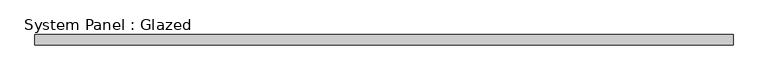
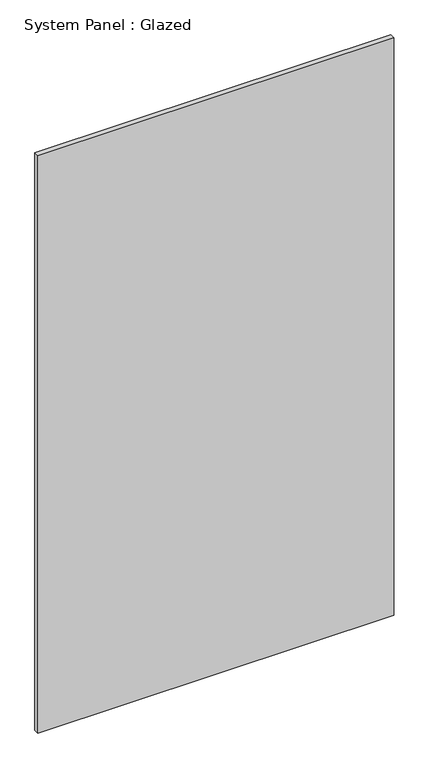
"""IFC4 building model written with IfcOpenShell, lengths in millimetres: plate geometry, System Panel : Glazed."""

from ifc_helpers import new_model, si_unit, origin, origin_with_axes, place, context, project, spatial, polyline, outline, extrude, source, transform, mapped, element, save


def system_panel_glazed_370bf902(model_context):
    return source(origin(), model_context, "Body", "SweptSolid", [
        extrude(outline(polyline([(850.9, 19.05), (-850.9, 19.05), (-850.9, 44.45), (850.9, 44.45), (850.9, 19.05)])), origin_with_axes(), (0.0, 0.0, 1.0), 2921.0),
    ])


if __name__ == "__main__":
    model = new_model("IFC4")
    model_context = context("Model", 3, world=origin())
    ifc_project = project(units=[si_unit("LENGTHUNIT", "METRE", prefix="MILLI")], contexts=[model_context])
    site = spatial("IfcSite", under=ifc_project)
    building = spatial("IfcBuilding", under=site)
    placement = place(None, origin())
    system_panel_glazed_shape = system_panel_glazed_370bf902(model_context)
    element("IfcPlate", 1, ObjectType="System Panel : Glazed", at=placement, inside=building, context=model_context, shape_type="MappedRepresentation", body=[
        mapped(system_panel_glazed_shape, transform((0.0, 0.0, 0.0), x_axis=(1.0, 0.0, 0.0), y_axis=(0.0, 1.0, 0.0), z_axis=(0.0, 0.0, 1.0))),
    ])
    save(model, "model.ifc")

# Revit data of these elements
# Type "System Panel : Glazed"
#   Construction Type Id = "GSP4R"
#   Analytic Construction = "1/8 in Pilkington single glazing"
#   Visual Light Transmittance = 0.9
#   Solar Heat Gain Coefficient = 0.86
#   Heat Transfer Coefficient (U) = 1.18115 BTU/(h·ft²·°F)
# Element 1 (IfcPlate, "System Panel : Glazed")
#   Materials on its faces: "Glass"
# Materials
#   "Glass": class "Glass", colour RGB 0 128 192, transparency 0.75, Description = "Soda Lime Glass", Cost = 0
